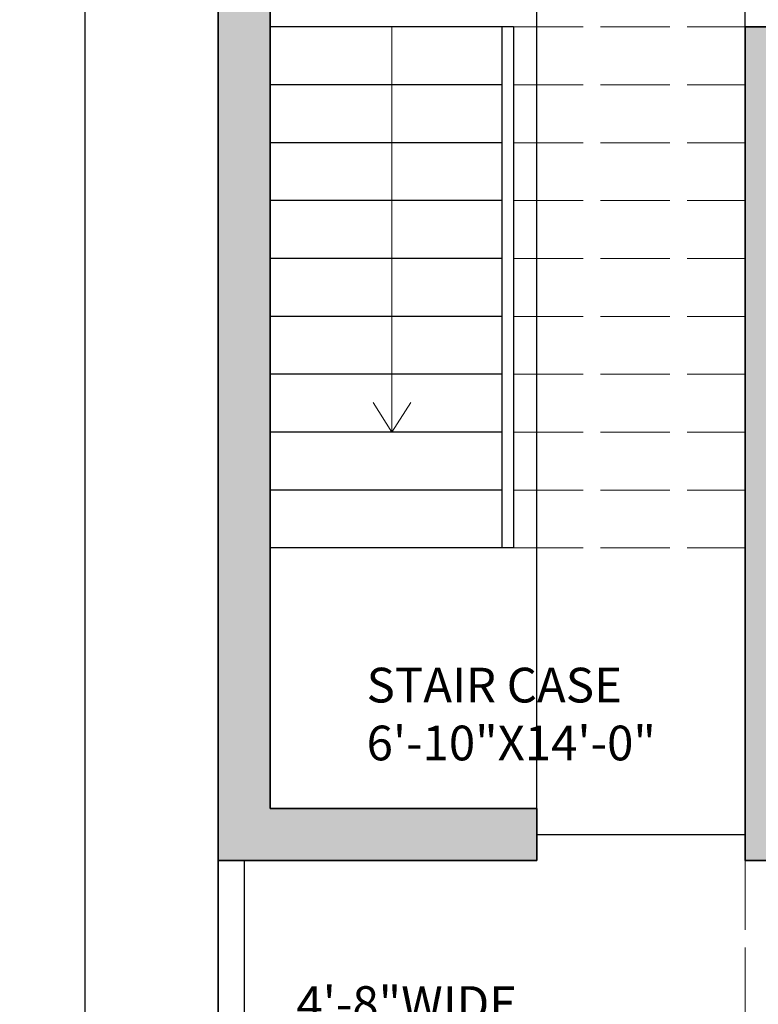
# Model space of a CAD drawing. Units: inches. Extents: x -16 to 587, y -783 to 64.
# Tile 2 of 14: x -16 to 111, y -697 to -527. Entities that reach past the tile are written whole.
import ezdxf

# ---------------------------------------------------------------- set-up
doc = ezdxf.new("R2010")
doc.units = ezdxf.units.IN
doc.header["$MEASUREMENT"] = 0
doc.linetypes.add('ACAD_ISO02W100', pattern=[15, 12, -3])
for name, color, linetype, lineweight in [('A-ANNO-DIMS', 2, 'Continuous', 18), ('A-ANNO-SYMB', 7, 'Continuous', 18), ('A-AREA-IDEN', 7, 'Continuous', 18), ('A-DOOR', 3, 'Continuous', 25), ('A-FLOR-OVHD', 8, 'ACAD_ISO02W100', 18), ('A-FLOR-STRS', 7, 'Continuous', 25), ('A-FLOR-STRS-OVHD', 7, 'ACAD_ISO02W100', 18), ('A-SITE-WALL', 7, 'Continuous', 30), ('A-WALL', 7, 'Continuous', 35), ('A-WALL-PATT', 23, 'Continuous', 13)]:
    doc.layers.add(name, color=color, linetype=linetype, lineweight=lineweight)
doc.styles.get("Standard").update_dxf_attribs({"font": 'arial.ttf'})
doc.dimstyles.get("Standard").update_dxf_attribs({"dimtxt": 0.18, "dimasz": 0.18, "dimexe": 0.18, "dimexo": 0.0625, "dimgap": 0.09, "dimtad": 0, "dimtih": 1, "dimtoh": 1, "dimdec": 0, "dimzin": 0, "dimdsep": 46, "dimlunit": 3, "dimtxsty": 'Standard', "dimcen": 0.09, "dimadec": 0, "dimazin": 0, "dimtfac": 1, "dimtdec": 0, "dimtofl": 0, "dimtmove": 0, "dimatfit": 3, "dimfxl": 1, "dimtolj": 1, "dimtzin": 0, "dimarcsym": 0})

# ---------------------------------------------------------------- blocks, each defined once
blk = doc.blocks.new('*D6')
at = {"layer": 'A-ANNO-DIMS', "color": 0, "lineweight": -2, "transparency": 16777216}
for p, q in [((18.02, 19.45), (-5.05, 19.45)), ((-4.87, 19.27), (-4.87, -355.9)), ((-4.87, -737.37), (-4.87, -362.21)), ((18.02, -737.55), (-5.05, -737.55))]:
    blk.add_line(p, q, dxfattribs=at)
at = {"layer": 'A-ANNO-DIMS', "color": 0, "transparency": 16777216}
for points in [[(-4.9, 19.27), (-4.84, 19.27), (-4.87, 19.45)], [(-4.9, -737.37), (-4.84, -737.37), (-4.87, -737.55)]]:
    blk.add_solid(points, dxfattribs=at)
at = {"layer": 'Defpoints', "color": 0, "transparency": 16777216}
for p in [(18.08, 19.45), (-4.87, -737.55), (18.08, -737.55)]:
    blk.add_point(p, dxfattribs=at)
at = {"layer": 'A-ANNO-DIMS', "color": 0, "transparency": 16777216, "insert": (-4.87, -359.05), "char_height": 6, "attachment_point": 5}
blk.add_mtext('\\A1;63\'-1"', dxfattribs=at)
blk = doc.blocks.new('STAIR-DIRECTION')
for p, q in [((3.25, 70), (3.25, 0)), ((3.25, 0), (0, 5.12)), ((3.25, 0), (6.51, 5.12))]:
    blk.add_line(p, q)
blk = doc.blocks.new('*D58')
at = {"layer": 'A-ANNO-DIMS', "color": 0, "lineweight": -2, "transparency": 16777216}
for p, q in [((73.08, -663.49), (73.08, 63.78)), ((73.26, 63.6), (90.75, 63.6)), ((108.9, 63.6), (91.41, 63.6)), ((109.08, -667.99), (109.08, 63.78))]:
    blk.add_line(p, q, dxfattribs=at)
at = {"layer": 'A-ANNO-DIMS', "color": 0, "transparency": 16777216}
for points in [[(73.26, 63.63), (73.26, 63.57), (73.08, 63.6)], [(108.9, 63.63), (108.9, 63.57), (109.08, 63.6)]]:
    blk.add_solid(points, dxfattribs=at)
at = {"layer": 'Defpoints', "color": 0, "transparency": 16777216}
for p in [(109.08, 63.6), (73.08, -663.55), (109.08, -668.05)]:
    blk.add_point(p, dxfattribs=at)
at = {"layer": 'A-ANNO-DIMS', "color": 0, "transparency": 16777216, "insert": (91.08, 63.6), "char_height": 0.18, "attachment_point": 5}
blk.add_mtext('\\A1;3\'-0"', dxfattribs=at)

msp = doc.modelspace()

# ---------------------------------------------------------------- hatches: boundary and pattern name
at = {"layer": 'A-WALL-PATT'}
h = msp.add_hatch(color=256, dxfattribs=at)
h.dxf.hatch_style = 1
h.paths.add_polyline_path([(137.08, -543.55), (137.08, -534.55), (118.08, -534.55), (118.08, -528.55), (109.08, -528.55), (109.08, -534.55), (109.08, -672.55), (118.08, -672.55), (118.08, -543.55)], flags=17)
h.paths.add_polyline_path([(27.08, -663.55), (27.08, -400.55), (73.08, -400.55), (73.08, -391.55), (27.08, -391.55), (27.08, 10.45), (48.75, 10.45), (171.08, 10.45), (171.08, -17.55), (180.08, -17.55), (180.08, 10.45), (228.08, 10.45), (228.08, -262.55), (206.41, -262.55), (118.08, -262.55), (118.08, -271.55), (228.08, -271.55), (228.08, -391.55), (154.08, -391.55), (154.08, -400.55), (228.08, -400.55), (228.08, -534.55), (209.08, -534.55), (209.08, -543.55), (237.08, -543.55), (237.08, 19.45), (18.08, 19.45), (18.08, -672.55), (73.08, -672.55), (73.08, -663.55)])
h.paths.add_polyline_path([(109.08, -486.55), (87.08, -486.55), (87.08, -495.55), (118.08, -495.55), (118.08, -400.55), (118.08, -391.55), (109.08, -391.55), (109.08, -400.55)], flags=17)

# ---------------------------------------------------------------- linework, layer by layer
at = {"layer": 'A-DOOR'}
msp.add_line((73.08, -668.05), (109.08, -668.05), dxfattribs=at)
at = {"layer": 'A-FLOR-OVHD'}
msp.add_line((109.08, -672.55), (109.08, -720.26), dxfattribs=at)
at = {"layer": 'A-FLOR-STRS'}
for p, q in [((69.08, -528.55), (27.08, -528.55)), ((67.08, -528.55), (67.08, -618.55)), ((69.08, -528.55), (69.08, -618.55)), ((67.08, -538.55), (27.08, -538.55)), ((67.08, -548.55), (27.08, -548.55)), ((67.08, -558.55), (27.08, -558.55)), ((67.08, -568.55), (27.08, -568.55)), ((67.08, -578.55), (27.08, -578.55)), ((67.08, -588.55), (27.08, -588.55)), ((67.08, -598.55), (27.08, -598.55)), ((67.08, -608.55), (27.08, -608.55)), ((69.08, -618.55), (27.08, -618.55))]:
    msp.add_line(p, q, dxfattribs=at)
at = {"layer": 'A-FLOR-STRS-OVHD'}
for p, q in [((69.08, -528.55), (109.08, -528.55)), ((69.08, -538.55), (109.08, -538.55)), ((69.08, -548.55), (109.08, -548.55)), ((69.08, -558.55), (109.08, -558.55)), ((69.08, -568.55), (109.08, -568.55)), ((69.08, -578.55), (109.08, -578.55)), ((69.08, -578.55), (109.08, -578.55)), ((69.08, -588.55), (109.08, -588.55)), ((69.08, -588.55), (109.08, -588.55)), ((69.08, -598.55), (109.08, -598.55)), ((69.08, -608.55), (109.08, -608.55)), ((69.08, -618.55), (109.08, -618.55))]:
    msp.add_line(p, q, dxfattribs=at)
at = {"layer": 'A-SITE-WALL'}
msp.add_line((22.58, -672.55), (22.58, -728.55), dxfattribs=at)
at = {"layer": 'A-WALL'}
for p, q in [((18.08, 19.45), (18.08, -737.55)), ((27.08, -400.55), (27.08, -663.55)), ((118.08, -528.55), (109.08, -528.55)), ((109.08, -528.55), (109.08, -534.55)), ((109.08, -534.55), (109.08, -672.55)), ((27.08, -663.55), (73.08, -663.55)), ((73.08, -663.55), (73.08, -672.55)), ((18.08, -672.55), (73.08, -672.55)), ((109.08, -672.55), (118.08, -672.55))]:
    msp.add_line(p, q, dxfattribs=at)

# ---------------------------------------------------------------- block references
at = {"layer": 'A-ANNO-SYMB'}
msp.add_blockref('STAIR-DIRECTION', (44.83, -598.55), dxfattribs=at)

# ---------------------------------------------------------------- texts
at = {"layer": 'A-AREA-IDEN', "char_height": 6, "attachment_point": 1}
for s, insert in [('STAIR CASE\\P6\'-10"X14\'-0"', (43.71, -639.25)), ('4\'-8"WIDE\\PFRONT SET BACK', (31.59, -694.26))]:
    msp.add_mtext(s, dxfattribs=dict(at, insert=insert))

# ---------------------------------------------------------------- dimensions: what is measured, and where the dimension line sits
at = {"layer": 'A-ANNO-DIMS'}
dim = msp.add_linear_dim(base=(109.08, 63.6), p1=(73.08, -663.55), p2=(109.08, -668.05), dimstyle='Standard', override={"dimdec": 1, "dimlfac": 1, "dimrnd": 0, "dimzin": 1, "dimdsep": 46, "dimlunit": 4, "dimfrac": 2}, dxfattribs=at)
dim.commit()
dim.dimension.update_dxf_attribs({"geometry": '*D58', "text_midpoint": (91.08, 63.6)})
dim = msp.add_linear_dim(base=(-4.87, -737.55), p1=(18.08, 19.45), p2=(18.08, -737.55), angle=90, dimstyle='Standard', override={"dimtxt": 6, "dimclrd": 0, "dimclre": 0, "dimclrt": 0}, dxfattribs=at)
dim.commit()
dim.dimension.update_dxf_attribs({"geometry": '*D6', "text_midpoint": (-4.87, -359.05)})

doc.saveas('drawing.dxf')
